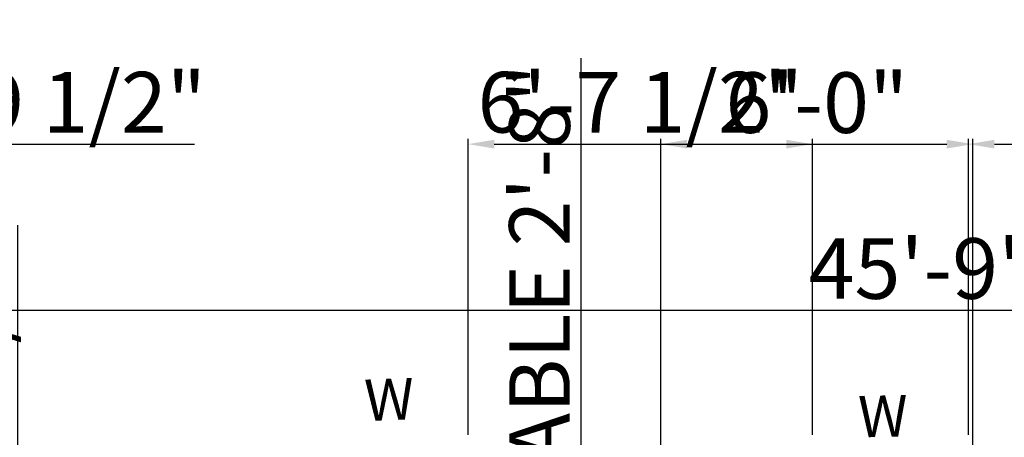
# Model space of a CAD drawing. Units: inches. Extents: x 2961 to 3748, y 1432 to 1961.
# Tile 7 of 9: x 3120 to 3348, y 1865 to 1961. Entities that reach past the tile are written whole.
import ezdxf
from ezdxf.enums import TextEntityAlignment as Align

# ---------------------------------------------------------------- set-up
doc = ezdxf.new("R2010")
doc.units = ezdxf.units.IN
doc.layers.add('A-ANNO-DIMS', color=2, linetype='Continuous', lineweight=18)
doc.layers.add('A-ANNO-TEXT', color=7, linetype='Continuous', lineweight=18)
doc.styles.get("Standard").update_dxf_attribs({"font": 'arial.ttf'})
doc.dimstyles.new('ISO-25', dxfattribs={"dimtxt": 14, "dimasz": 6, "dimexe": 1.25, "dimexo": 0.625, "dimtad": 1, "dimlunit": 3, "dimtxsty": 'Standard', "dimcen": 2.5, "dimadec": 0, "dimazin": 0, "dimtfac": 1, "dimtmove": 0, "dimatfit": 3, "dimfxl": 1, "dimarcsym": 0})

# ---------------------------------------------------------------- blocks, each defined once
blk = doc.blocks.new('*D14')
at = {"layer": 'A-ANNO-DIMS', "color": 0, "lineweight": -2, "transparency": 16777216}
for p, q in [((3054.27, 1865.26), (3054.27, 1895.31)), ((3060.27, 1894.06), (3597.27, 1894.06)), ((3603.27, 1865.26), (3603.27, 1895.31))]:
    blk.add_line(p, q, dxfattribs=at)
at = {"layer": 'A-ANNO-DIMS', "color": 0, "transparency": 16777216}
for points in [[(3060.27, 1895.06), (3060.27, 1893.06), (3054.27, 1894.06)], [(3597.27, 1895.06), (3597.27, 1893.06), (3603.27, 1894.06)]]:
    blk.add_solid(points, dxfattribs=at)
at = {"layer": 'Defpoints', "color": 0, "transparency": 16777216}
for p in [(3603.27, 1894.06), (3054.27, 1864.64), (3603.27, 1864.64)]:
    blk.add_point(p, dxfattribs=at)
at = {"layer": 'A-ANNO-DIMS', "color": 0, "transparency": 16777216, "insert": (3328.77, 1901.84), "char_height": 14, "attachment_point": 5}
blk.add_mtext('45\'-9"', dxfattribs=at)
blk = doc.blocks.new('*D30')
at = {"layer": 'A-ANNO-DIMS', "color": 0, "lineweight": -2, "transparency": 16777216}
for p, q in [((3249.85, 1839.99), (3249.85, 1952.2)), ((3245.67, 1839.99), (3251.1, 1839.99)), ((3249.85, 1813.95), (3249.85, 1833.99)), ((3245.67, 1807.95), (3251.1, 1807.95))]:
    blk.add_line(p, q, dxfattribs=at)
at = {"layer": 'A-ANNO-DIMS', "color": 0, "transparency": 16777216}
for points in [[(3248.85, 1833.99), (3250.85, 1833.99), (3249.85, 1839.99)], [(3248.85, 1813.95), (3250.85, 1813.95), (3249.85, 1807.95)]]:
    blk.add_solid(points, dxfattribs=at)
at = {"layer": 'Defpoints', "color": 0, "transparency": 16777216}
for p in [(3245.04, 1839.99), (3249.85, 1839.99), (3245.04, 1807.95)]:
    blk.add_point(p, dxfattribs=at)
at = {"layer": 'A-ANNO-DIMS', "color": 0, "transparency": 16777216, "insert": (3242.07, 1899.09), "char_height": 14, "attachment_point": 5, "rotation": 90}
blk.add_mtext('TABLE 2\'-8"', dxfattribs=at)
blk = doc.blocks.new('*D46')
at = {"layer": 'A-ANNO-DIMS', "color": 0, "lineweight": -2, "transparency": 16777216}
for p, q in [((3119.82, 1773.04), (3119.82, 1913.63)), ((3116.76, 1773.04), (3121.07, 1773.04)), ((3119.82, 1754.49), (3119.82, 1767.04)), ((3116.76, 1748.49), (3121.07, 1748.49))]:
    blk.add_line(p, q, dxfattribs=at)
at = {"layer": 'A-ANNO-DIMS', "color": 0, "transparency": 16777216}
for points in [[(3118.82, 1767.04), (3120.82, 1767.04), (3119.82, 1773.04)], [(3118.82, 1754.49), (3120.82, 1754.49), (3119.82, 1748.49)]]:
    blk.add_solid(points, dxfattribs=at)
at = {"layer": 'Defpoints', "color": 0, "transparency": 16777216}
for p in [(3116.13, 1773.04), (3119.82, 1773.04), (3116.13, 1748.49)]:
    blk.add_point(p, dxfattribs=at)
at = {"layer": 'A-ANNO-DIMS', "color": 0, "transparency": 16777216, "insert": (3111.95, 1846.34), "char_height": 14, "attachment_point": 5, "rotation": 90}
blk.add_mtext('BASIN 2\'-0 1/2"', dxfattribs=at)
blk = doc.blocks.new('*D54')
at = {"layer": 'A-ANNO-DIMS', "color": 0, "lineweight": -2, "transparency": 16777216}
for p, q in [((3223.8, 1865.26), (3223.8, 1933.63)), ((3229.8, 1932.38), (3297.27, 1932.38)), ((3303.27, 1865.26), (3303.27, 1933.63))]:
    blk.add_line(p, q, dxfattribs=at)
at = {"layer": 'A-ANNO-DIMS', "color": 0, "transparency": 16777216}
for points in [[(3229.8, 1933.38), (3229.8, 1931.38), (3223.8, 1932.38)], [(3297.27, 1933.38), (3297.27, 1931.38), (3303.27, 1932.38)]]:
    blk.add_solid(points, dxfattribs=at)
at = {"layer": 'Defpoints', "color": 0, "transparency": 16777216}
for p in [(3303.27, 1932.38), (3223.8, 1864.64), (3303.27, 1864.64)]:
    blk.add_point(p, dxfattribs=at)
at = {"layer": 'A-ANNO-DIMS', "color": 0, "transparency": 16777216, "insert": (3263.53, 1940.24), "char_height": 14, "attachment_point": 5}
blk.add_mtext('6\'-7 1/2"', dxfattribs=at)
blk = doc.blocks.new('*D55')
at = {"layer": 'A-ANNO-DIMS', "color": 0, "lineweight": -2, "transparency": 16777216}
for p, q in [((3339.27, 1865.26), (3339.27, 1933.63)), ((3345.27, 1932.38), (3429.27, 1932.38)), ((3435.27, 1865.26), (3435.27, 1933.63))]:
    blk.add_line(p, q, dxfattribs=at)
at = {"layer": 'A-ANNO-DIMS', "color": 0, "transparency": 16777216}
for points in [[(3345.27, 1933.38), (3345.27, 1931.38), (3339.27, 1932.38)], [(3429.27, 1933.38), (3429.27, 1931.38), (3435.27, 1932.38)]]:
    blk.add_solid(points, dxfattribs=at)
at = {"layer": 'Defpoints', "color": 0, "transparency": 16777216}
for p in [(3435.27, 1932.38), (3339.27, 1864.64), (3435.27, 1864.64)]:
    blk.add_point(p, dxfattribs=at)
at = {"layer": 'A-ANNO-DIMS', "color": 0, "transparency": 16777216, "insert": (3387.27, 1940.15), "char_height": 14, "attachment_point": 5}
blk.add_mtext('8\'-0"', dxfattribs=at)
blk = doc.blocks.new('*D69')
at = {"layer": 'A-ANNO-DIMS', "color": 0, "lineweight": -2, "transparency": 16777216}
for p, q in [((3268.27, 1646.26), (3268.27, 1933.63)), ((3274.27, 1932.38), (3334.27, 1932.38)), ((3340.27, 1646.26), (3340.27, 1933.63))]:
    blk.add_line(p, q, dxfattribs=at)
at = {"layer": 'A-ANNO-DIMS', "color": 0, "transparency": 16777216}
for points in [[(3274.27, 1933.38), (3274.27, 1931.38), (3268.27, 1932.38)], [(3334.27, 1933.38), (3334.27, 1931.38), (3340.27, 1932.38)]]:
    blk.add_solid(points, dxfattribs=at)
at = {"layer": 'Defpoints', "color": 0, "transparency": 16777216}
for p in [(3340.27, 1932.38), (3268.27, 1645.64), (3340.27, 1645.64)]:
    blk.add_point(p, dxfattribs=at)
at = {"layer": 'A-ANNO-DIMS', "color": 0, "transparency": 16777216, "insert": (3304.27, 1940.15), "char_height": 14, "attachment_point": 5}
blk.add_mtext('6\'-0"', dxfattribs=at)
blk = doc.blocks.new('*D82')
at = {"layer": 'A-ANNO-DIMS', "color": 0, "lineweight": -2, "transparency": 16777216}
for p, q in [((3063.27, 1542.49), (3063.27, 1933.63)), ((3069.27, 1932.38), (3078.82, 1932.38)), ((3084.82, 1542.49), (3084.82, 1933.63)), ((3084.82, 1932.38), (3160.59, 1932.38))]:
    blk.add_line(p, q, dxfattribs=at)
at = {"layer": 'A-ANNO-DIMS', "color": 0, "transparency": 16777216}
for points in [[(3069.27, 1933.38), (3069.27, 1931.38), (3063.27, 1932.38)], [(3078.82, 1933.38), (3078.82, 1931.38), (3084.82, 1932.38)]]:
    blk.add_solid(points, dxfattribs=at)
at = {"layer": 'Defpoints', "color": 0, "transparency": 16777216}
for p in [(3084.82, 1932.38), (3063.27, 1541.87), (3084.82, 1541.87)]:
    blk.add_point(p, dxfattribs=at)
at = {"layer": 'A-ANNO-DIMS', "color": 0, "transparency": 16777216, "insert": (3125.71, 1940.24), "char_height": 14, "attachment_point": 5}
blk.add_mtext('1\'-9 1/2"', dxfattribs=at)

msp = doc.modelspace()

# ---------------------------------------------------------------- texts
at = {"layer": 'A-ANNO-TEXT'}
for rotation, p in [(2.15165, (3205.761, 1868.627)), (1.05867, (3319.628, 1864.755))]:
    msp.add_text('W', height=9.571, rotation=rotation, dxfattribs=at).set_placement(p, align=Align.CENTER)

# ---------------------------------------------------------------- dimensions: what is measured, and where the dimension line sits
at = {"layer": 'A-ANNO-DIMS'}
for base, p1, p2, override, picture, middle in [((3084.825, 1932.38), (3063.267, 1541.867), (3084.825, 1541.867), {"dimdec": 1, "dimlfac": 1, "dimrnd": 0, "dimzin": 1, "dimdsep": 46, "dimlunit": 4, "dimfrac": 2}, '*D82', (3125.71, 1940.244)), ((3303.267, 1932.38), (3223.801, 1864.639), (3303.267, 1864.639), {"dimdec": 1, "dimlfac": 1, "dimrnd": 0, "dimzin": 1, "dimdsep": 46, "dimlunit": 4, "dimfrac": 2}, '*D54', (3263.534, 1940.244)), ((3340.267, 1932.38), (3268.267, 1645.639), (3340.267, 1645.639), {"dimdec": 1, "dimlfac": 1, "dimrnd": 0, "dimzin": 1, "dimdsep": 46, "dimlunit": 4, "dimfrac": 2}, '*D69', (3304.267, 1940.153)), ((3435.267, 1932.38), (3339.267, 1864.639), (3435.267, 1864.639), {"dimdec": 1, "dimlfac": 1, "dimrnd": 0, "dimzin": 1, "dimdsep": 46, "dimlunit": 4, "dimfrac": 2}, '*D55', (3387.267, 1940.153)), ((3603.267, 1894.063), (3054.267, 1864.639), (3603.267, 1864.639), {"dimclrd": 0, "dimclre": 0, "dimclrt": 0}, '*D14', (3328.767, 1901.836))]:
    dim = msp.add_linear_dim(base=base, p1=p1, p2=p2, dimstyle='ISO-25', override=override, dxfattribs=at)
    dim.commit()
    dim.dimension.update_dxf_attribs({"geometry": picture, "text_midpoint": middle})
for base, p1, p2, text, picture, middle in [((3249.847, 1839.987), (3245.042, 1807.952), (3245.042, 1839.987), 'TABLE <>', '*D30', (3242.074, 1899.093)), ((3119.818, 1773.04), (3116.135, 1748.489), (3116.135, 1773.04), 'BASIN <>', '*D46', (3111.954, 1846.336))]:
    dim = msp.add_linear_dim(base=base, p1=p1, p2=p2, angle=90, text=text, dimstyle='ISO-25', override={"dimdec": 1, "dimlfac": 1, "dimrnd": 0, "dimzin": 1, "dimdsep": 46, "dimlunit": 4, "dimfrac": 2}, dxfattribs=at)
    dim.commit()
    dim.dimension.update_dxf_attribs({"geometry": picture, "text_midpoint": middle})

doc.saveas('drawing.dxf')
